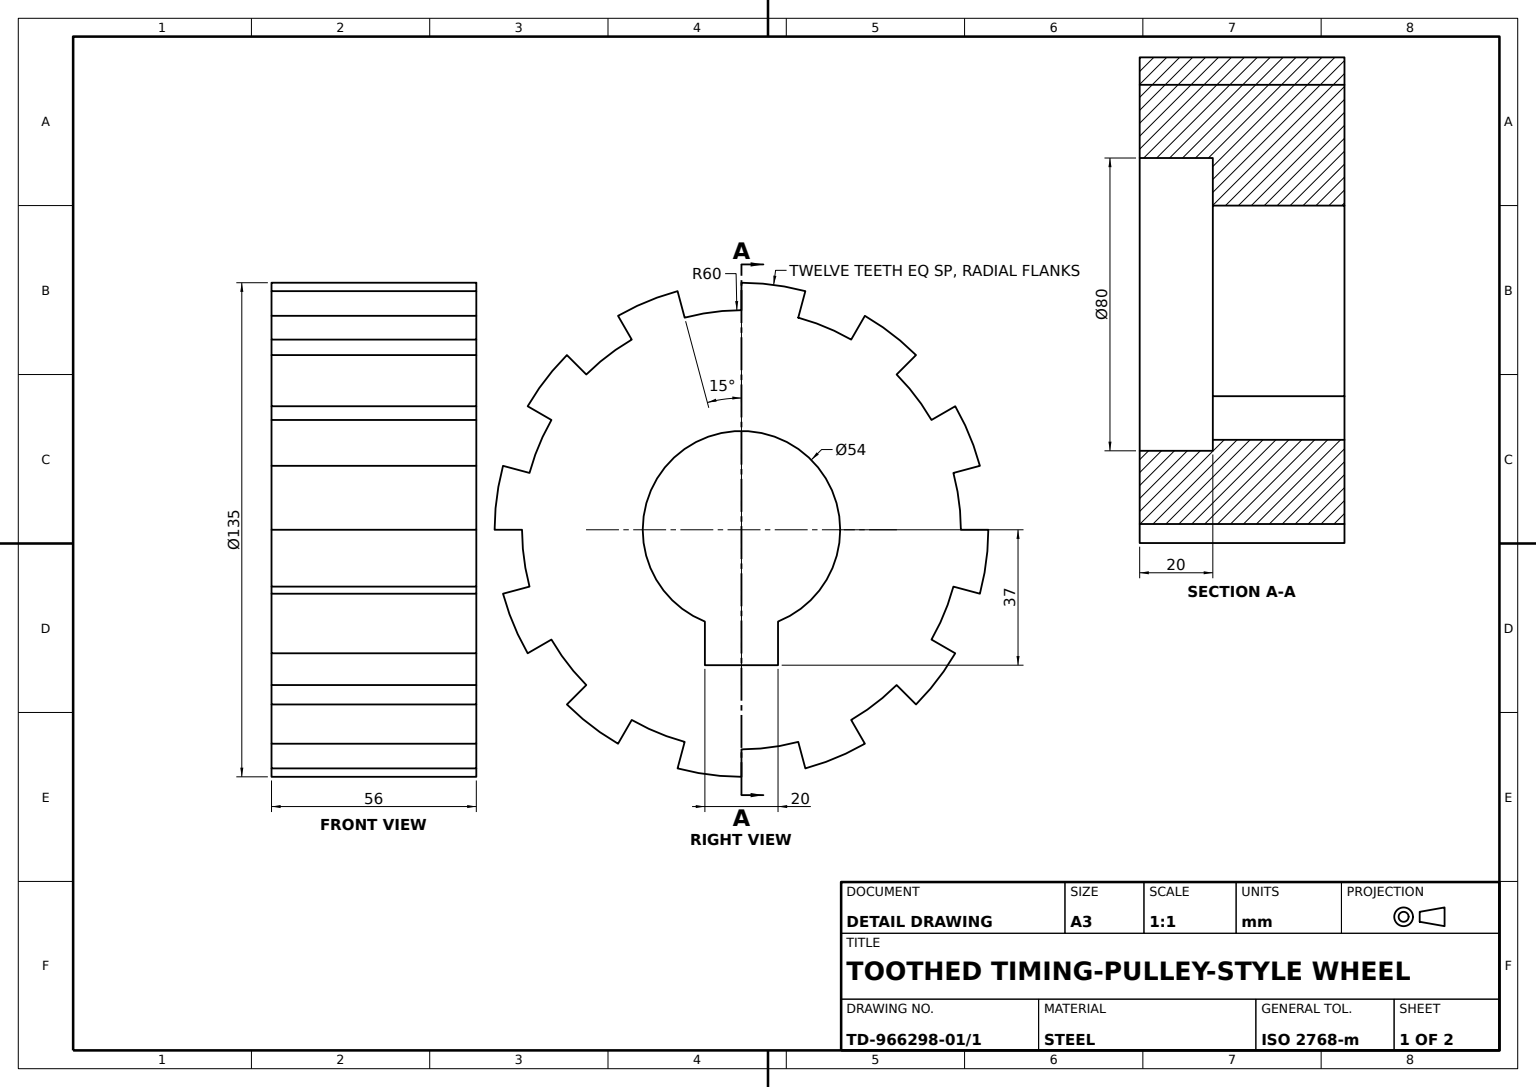
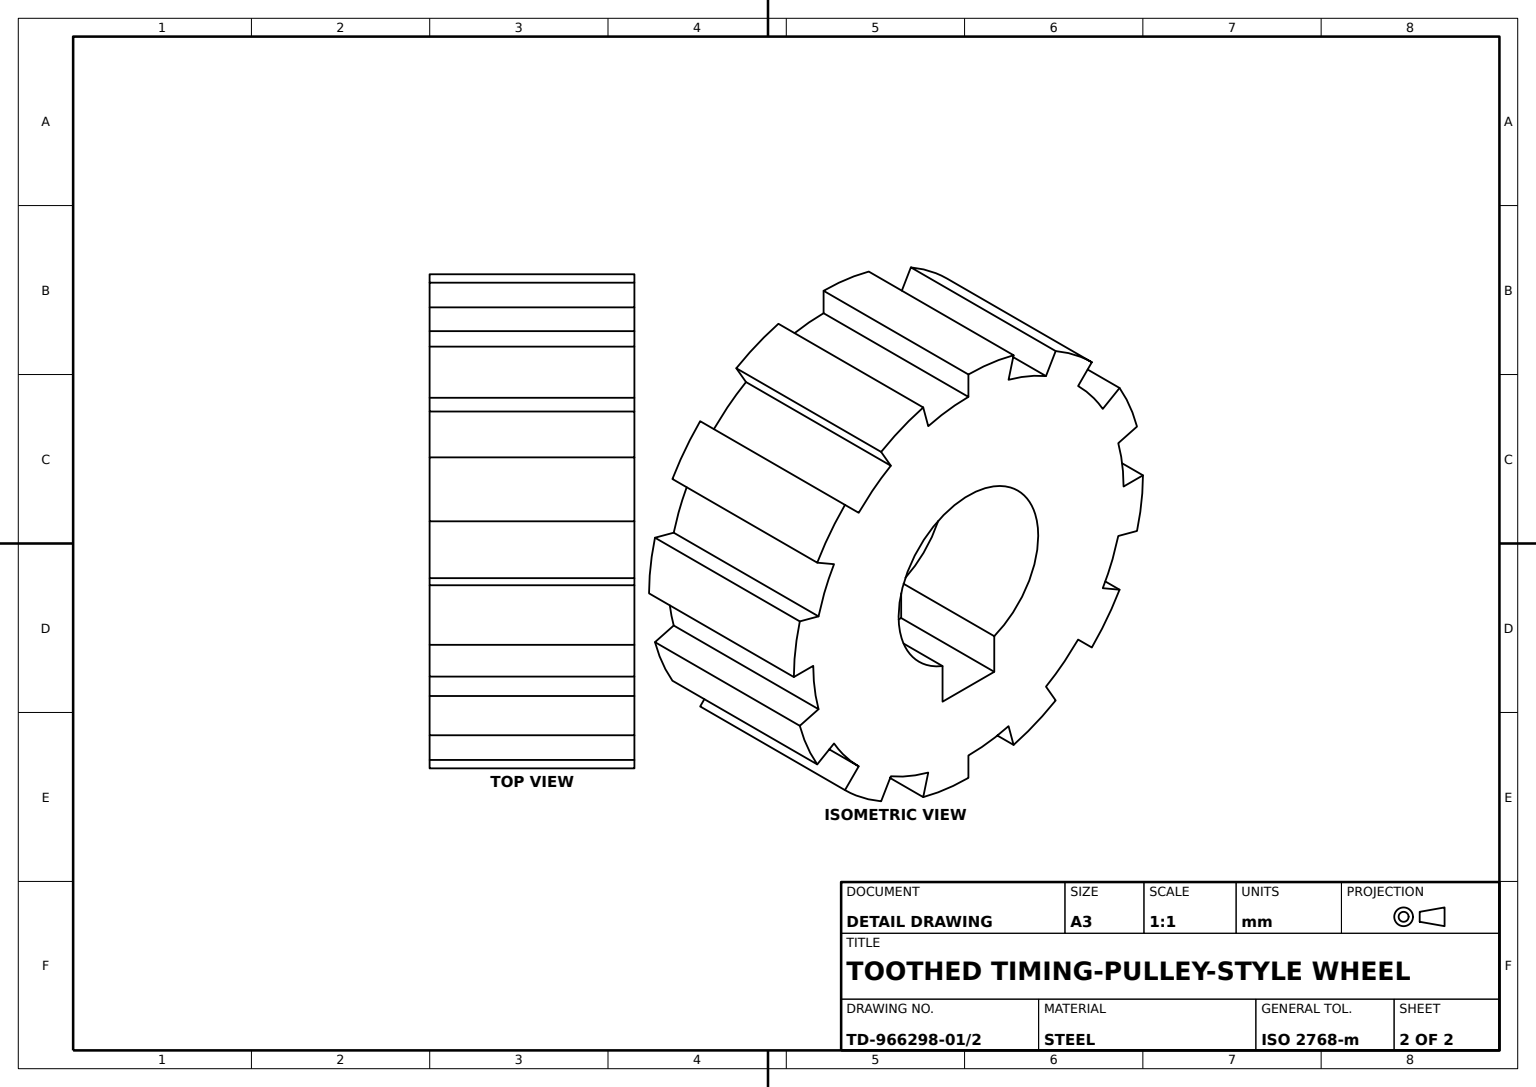
from build123d import *

# Parameters (mm, degrees)
GEAR_BODY_12T_DEPTH  = 56
FACE_RECESS_SKETCH_R = 40
FACE_RECESS_80_DEPTH = 20
BORE_CUT_DEPTH       = 36


with BuildPart() as part:
    # Gear Tooth Profile Sketch → Gear Body 12T (new body)
    with BuildSketch(Plane.XY):
        with BuildLine():
            Line((-15.529142706, 57.955549577), (-17.470285544, 65.199993275))
            ThreePointArc((-17.470285544, 65.199993275), (-8.810517975, 66.922528143), (0, 67.5))
            Line((0, 67.5), (0, 60))
            ThreePointArc((0, 60), (7.831571533, 59.486691682), (15.529142706, 57.955549577))
            Line((15.529142706, 57.955549577), (17.470285544, 65.199993275))
            ThreePointArc((17.470285544, 65.199993275), (25.831131685, 62.361868445), (33.75, 58.456714755))
            Line((33.75, 58.456714755), (30, 51.961524227))
            ThreePointArc((30, 51.961524227), (36.525685741, 47.601200417), (42.426406871, 42.426406871))
            Line((42.426406871, 42.426406871), (47.72970773, 47.72970773))
            ThreePointArc((47.72970773, 47.72970773), (53.55135047, 41.091396458), (58.456714755, 33.75))
            Line((58.456714755, 33.75), (51.961524227, 30))
            ThreePointArc((51.961524227, 30), (55.432771951, 22.961005942), (57.955549577, 15.529142706))
            Line((57.955549577, 15.529142706), (65.199993275, 17.470285544))
            ThreePointArc((65.199993275, 17.470285544), (66.922528143, 8.810517975), (67.5, 0))
            Line((67.5, 0), (60, 0))
            ThreePointArc((60, 0), (59.486691682, -7.831571533), (57.955549577, -15.529142706))
            Line((57.955549577, -15.529142706), (65.199993275, -17.470285544))
            ThreePointArc((65.199993275, -17.470285544), (62.361868445, -25.831131685), (58.456714755, -33.75))
            Line((58.456714755, -33.75), (51.961524227, -30))
            ThreePointArc((51.961524227, -30), (47.601200417, -36.525685741), (42.426406871, -42.426406871))
            Line((42.426406871, -42.426406871), (47.72970773, -47.72970773))
            ThreePointArc((47.72970773, -47.72970773), (41.091396458, -53.55135047), (33.75, -58.456714755))
            Line((33.75, -58.456714755), (30, -51.961524227))
            ThreePointArc((30, -51.961524227), (22.961005942, -55.432771951), (15.529142706, -57.955549577))
            Line((15.529142706, -57.955549577), (17.470285544, -65.199993275))
            ThreePointArc((17.470285544, -65.199993275), (8.810517975, -66.922528143), (0, -67.5))
            Line((0, -67.5), (0, -60))
            ThreePointArc((0, -60), (-7.831571533, -59.486691682), (-15.529142706, -57.955549577))
            Line((-15.529142706, -57.955549577), (-17.470285544, -65.199993275))
            ThreePointArc((-17.470285544, -65.199993275), (-25.831131685, -62.361868445), (-33.75, -58.456714755))
            Line((-33.75, -58.456714755), (-30, -51.961524227))
            ThreePointArc((-30, -51.961524227), (-36.525685741, -47.601200417), (-42.426406871, -42.426406871))
            Line((-42.426406871, -42.426406871), (-47.72970773, -47.72970773))
            ThreePointArc((-47.72970773, -47.72970773), (-53.55135047, -41.091396458), (-58.456714755, -33.75))
            Line((-58.456714755, -33.75), (-51.961524227, -30))
            ThreePointArc((-51.961524227, -30), (-55.432771951, -22.961005942), (-57.955549577, -15.529142706))
            Line((-57.955549577, -15.529142706), (-65.199993275, -17.470285544))
            ThreePointArc((-65.199993275, -17.470285544), (-66.922528143, -8.810517975), (-67.5, 0))
            Line((-67.5, 0), (-60, 0))
            ThreePointArc((-60, 0), (-59.486691682, 7.831571533), (-57.955549577, 15.529142706))
            Line((-57.955549577, 15.529142706), (-65.199993275, 17.470285544))
            ThreePointArc((-65.199993275, 17.470285544), (-62.361868445, 25.831131685), (-58.456714755, 33.75))
            Line((-58.456714755, 33.75), (-51.961524227, 30))
            ThreePointArc((-51.961524227, 30), (-47.601200417, 36.525685741), (-42.426406871, 42.426406871))
            Line((-42.426406871, 42.426406871), (-47.72970773, 47.72970773))
            ThreePointArc((-47.72970773, 47.72970773), (-41.091396458, 53.55135047), (-33.75, 58.456714755))
            Line((-33.75, 58.456714755), (-30, 51.961524227))
            ThreePointArc((-30, 51.961524227), (-22.961005942, 55.432771951), (-15.529142706, 57.955549577))
        make_face()
    extrude(amount=-GEAR_BODY_12T_DEPTH)

    # Face Recess Sketch → Face Recess Ø80 (cut)
    with BuildSketch(Plane.XY):
        Circle(FACE_RECESS_SKETCH_R)
    extrude(amount=-FACE_RECESS_80_DEPTH, mode=Mode.SUBTRACT)

    # Bore Profile Sketch → Bore Cut (cut)
    with BuildSketch(Plane.XY.offset(-20)):
        with BuildLine():
            Line((0, -37), (10, -37))
            Line((10, -37), (10, -25.079872408))
            ThreePointArc((10, -25.079872408), (0, 27), (-10, -25.079872408))
            Line((-10, -25.079872408), (-10, -37))
            Line((-10, -37), (0, -37))
        make_face()
    extrude(amount=-BORE_CUT_DEPTH, mode=Mode.SUBTRACT)


solid = part.part
